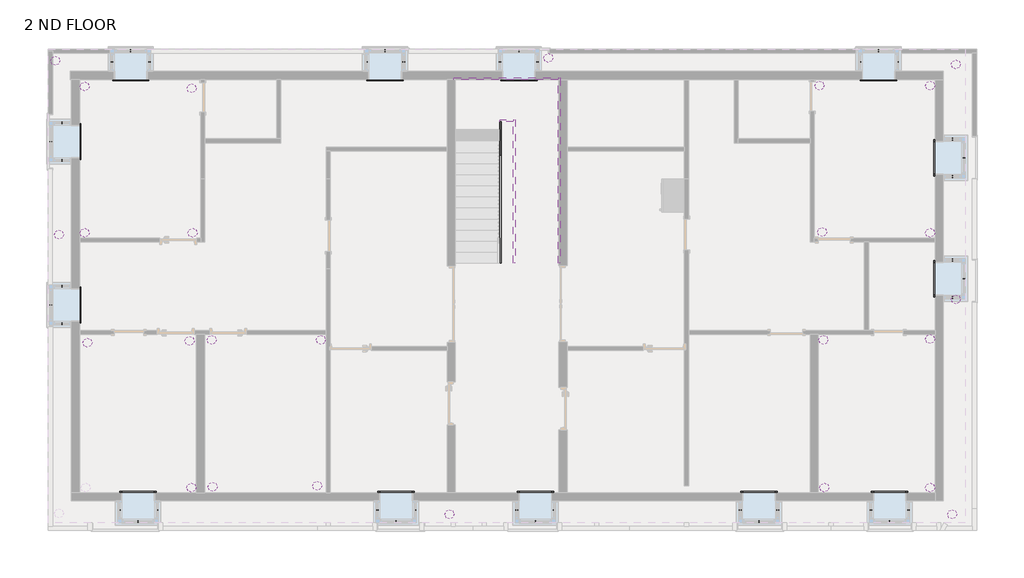
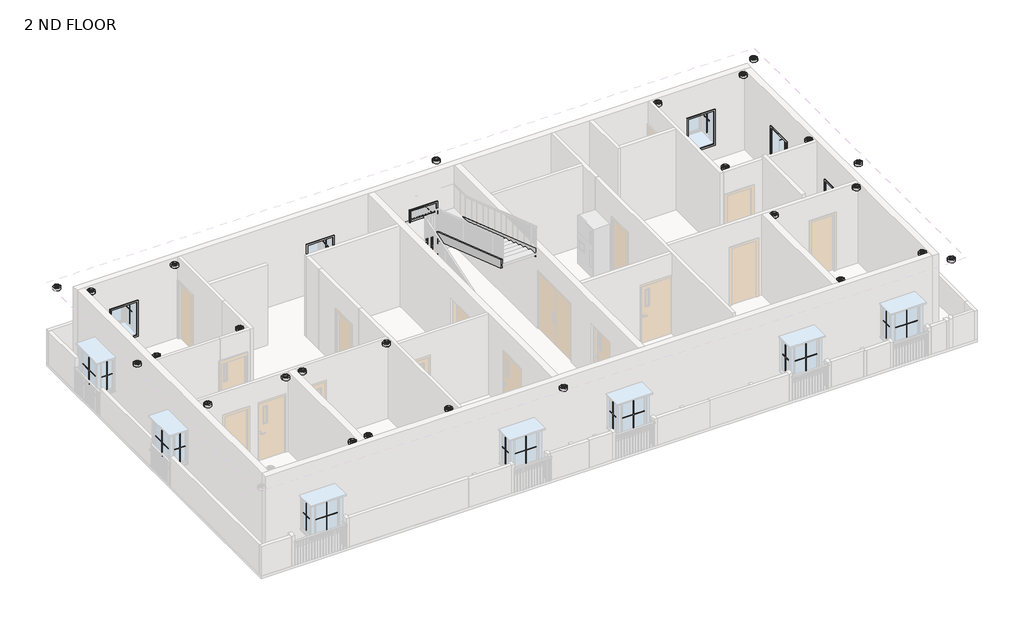
# One storey, part 7 of 7: 52 proxies, 26 light fixtures, 6 members.
"""IFC4 building model written with IfcOpenShell, lengths in millimetres."""

from ifc_helpers import new_model, si_unit, frame, origin, place, context, project, spatial, polyline, outline, extrude, transform, mapped, element, save
from components import muntin_pattern_2x2_muntin_pattern_2x2_95b57395, muntin_pattern_2x2_muntin_pattern_2x2_f03ab90d, trim_window_interior_flat_picture_frame_e50cf7ae, ceiling_light_flat_round_60w_120v_7c4c2a52

model = new_model("IFC4")

# Units and contexts
model_context = context("Model", 3, world=origin())
ifc_project = project(units=[si_unit("LENGTHUNIT", "METRE", prefix="MILLI")], contexts=[model_context])

# Site, building, storey
site = spatial("IfcSite", under=ifc_project)
building = spatial("IfcBuilding", under=site)
storey = spatial("IfcBuildingStorey", under=building, Name="2 ND FLOOR", Elevation=6400.8)

# Proxies
placement = place(None, origin())
muntin_pattern_2x2_muntin_pattern_2x2_shape = muntin_pattern_2x2_muntin_pattern_2x2_95b57395(model_context)
element("IfcBuildingElementProxy", 1, Name="Muntin Pattern_2x2 : Muntin Pattern_2x2", ObjectType="Muntin Pattern_2x2 : Muntin Pattern_2x2", at=placement, inside=storey, context=model_context, shape_type="MappedRepresentation", body=[
    mapped(muntin_pattern_2x2_muntin_pattern_2x2_shape, transform((-10814.9987925, 8428.7317329, 7131.05), x_axis=(1.0, 0.0, 0.0), y_axis=(0.0, 1.0, 0.0), z_axis=(0.0, 0.0, 1.0))),
])
element("IfcBuildingElementProxy", 2, Name="Muntin Pattern_2x2 : Muntin Pattern_2x2", ObjectType="Muntin Pattern_2x2 : Muntin Pattern_2x2", at=placement, inside=storey, context=model_context, shape_type="MappedRepresentation", body=[
    mapped(muntin_pattern_2x2_muntin_pattern_2x2_shape, transform((-3791.8987998, 8428.7317329, 7131.05), x_axis=(1.0, 0.0, 0.0), y_axis=(0.0, 1.0, 0.0), z_axis=(0.0, 0.0, 1.0))),
])
element("IfcBuildingElementProxy", 3, Name="Muntin Pattern_2x2 : Muntin Pattern_2x2", ObjectType="Muntin Pattern_2x2 : Muntin Pattern_2x2", at=placement, inside=storey, context=model_context, shape_type="MappedRepresentation", body=[
    mapped(muntin_pattern_2x2_muntin_pattern_2x2_shape, transform((-96.7067989, 8428.7317329, 7131.05), x_axis=(1.0, 0.0, 0.0), y_axis=(0.0, 1.0, 0.0), z_axis=(0.0, 0.0, 1.0))),
])
element("IfcBuildingElementProxy", 4, Name="Muntin Pattern_2x2 : Muntin Pattern_2x2", ObjectType="Muntin Pattern_2x2 : Muntin Pattern_2x2", at=placement, inside=storey, context=model_context, shape_type="MappedRepresentation", body=[
    mapped(muntin_pattern_2x2_muntin_pattern_2x2_shape, transform((9835.2012075, 8428.7317329, 7131.05), x_axis=(1.0, 0.0, 0.0), y_axis=(0.0, 1.0, 0.0), z_axis=(0.0, 0.0, 1.0))),
])
element("IfcBuildingElementProxy", 5, Name="Muntin Pattern_2x2 : Muntin Pattern_2x2", ObjectType="Muntin Pattern_2x2 : Muntin Pattern_2x2", at=placement, inside=storey, context=model_context, shape_type="MappedRepresentation", body=[
    mapped(muntin_pattern_2x2_muntin_pattern_2x2_shape, transform((-10611.7987958, -4582.4182193, 7131.05), x_axis=(-1.0, 0.0, 0.0), y_axis=(0.0, -1.0, 0.0), z_axis=(0.0, 0.0, 1.0))),
])
element("IfcBuildingElementProxy", 6, Name="Muntin Pattern_2x2 : Muntin Pattern_2x2", ObjectType="Muntin Pattern_2x2 : Muntin Pattern_2x2", at=placement, inside=storey, context=model_context, shape_type="MappedRepresentation", body=[
    mapped(muntin_pattern_2x2_muntin_pattern_2x2_shape, transform((-3487.0987998, -4582.4182193, 7131.05), x_axis=(-1.0, 0.0, 0.0), y_axis=(0.0, -1.0, 0.0), z_axis=(0.0, 0.0, 1.0))),
])
element("IfcBuildingElementProxy", 7, Name="Muntin Pattern_2x2 : Muntin Pattern_2x2", ObjectType="Muntin Pattern_2x2 : Muntin Pattern_2x2", at=placement, inside=storey, context=model_context, shape_type="MappedRepresentation", body=[
    mapped(muntin_pattern_2x2_muntin_pattern_2x2_shape, transform((360.4932011, -4582.4182193, 7131.05), x_axis=(-1.0, 0.0, 0.0), y_axis=(0.0, -1.0, 0.0), z_axis=(0.0, 0.0, 1.0))),
])
element("IfcBuildingElementProxy", 8, Name="Muntin Pattern_2x2 : Muntin Pattern_2x2", ObjectType="Muntin Pattern_2x2 : Muntin Pattern_2x2", at=placement, inside=storey, context=model_context, shape_type="MappedRepresentation", body=[
    mapped(muntin_pattern_2x2_muntin_pattern_2x2_shape, transform((6533.2012079, -4582.4182193, 7131.05), x_axis=(-1.0, 0.0, 0.0), y_axis=(0.0, -1.0, 0.0), z_axis=(0.0, 0.0, 1.0))),
])
element("IfcBuildingElementProxy", 9, Name="Muntin Pattern_2x2 : Muntin Pattern_2x2", ObjectType="Muntin Pattern_2x2 : Muntin Pattern_2x2", at=placement, inside=storey, context=model_context, shape_type="MappedRepresentation", body=[
    mapped(muntin_pattern_2x2_muntin_pattern_2x2_shape, transform((10140.0012075, -4582.4182193, 7131.05), x_axis=(-1.0, 0.0, 0.0), y_axis=(0.0, -1.0, 0.0), z_axis=(0.0, 0.0, 1.0))),
])
element("IfcBuildingElementProxy", 10, Name="Muntin Pattern_2x2 : Muntin Pattern_2x2", ObjectType="Muntin Pattern_2x2 : Muntin Pattern_2x2", at=placement, inside=storey, context=model_context, shape_type="MappedRepresentation", body=[
    mapped(muntin_pattern_2x2_muntin_pattern_2x2_shape, transform((12194.2262075, 2126.3567332, 7131.05), x_axis=(0.0, -1.0, 0.0), y_axis=(1.0, 0.0, 0.0), z_axis=(0.0, 0.0, 1.0))),
])
element("IfcBuildingElementProxy", 11, Name="Muntin Pattern_2x2 : Muntin Pattern_2x2", ObjectType="Muntin Pattern_2x2 : Muntin Pattern_2x2", at=placement, inside=storey, context=model_context, shape_type="MappedRepresentation", body=[
    mapped(muntin_pattern_2x2_muntin_pattern_2x2_shape, transform((12194.2262075, 5469.631733, 7131.05), x_axis=(0.0, -1.0, 0.0), y_axis=(1.0, 0.0, 0.0), z_axis=(0.0, 0.0, 1.0))),
])
element("IfcBuildingElementProxy", 12, Name="Muntin Pattern_2x2 : Muntin Pattern_2x2", ObjectType="Muntin Pattern_2x2 : Muntin Pattern_2x2", at=placement, inside=storey, context=model_context, shape_type="MappedRepresentation", body=[
    mapped(muntin_pattern_2x2_muntin_pattern_2x2_shape, transform((-13021.6237925, 1402.4567334, 7131.05), x_axis=(0.0, 1.0, 0.0), y_axis=(-1.0, 0.0, 0.0), z_axis=(0.0, 0.0, 1.0))),
])
element("IfcBuildingElementProxy", 13, Name="Muntin Pattern_2x2 : Muntin Pattern_2x2", ObjectType="Muntin Pattern_2x2 : Muntin Pattern_2x2", at=placement, inside=storey, context=model_context, shape_type="MappedRepresentation", body=[
    mapped(muntin_pattern_2x2_muntin_pattern_2x2_shape, transform((-13021.6237925, 5917.3067329, 7131.05), x_axis=(0.0, 1.0, 0.0), y_axis=(-1.0, 0.0, 0.0), z_axis=(0.0, 0.0, 1.0))),
])
muntin_pattern_2x2_muntin_pattern_2x2_2_shape = muntin_pattern_2x2_muntin_pattern_2x2_f03ab90d(model_context)
element("IfcBuildingElementProxy", 14, Name="Muntin Pattern_2x2 : Muntin Pattern_2x2", ObjectType="Muntin Pattern_2x2 : Muntin Pattern_2x2", at=placement, inside=storey, context=model_context, shape_type="MappedRepresentation", body=[
    mapped(muntin_pattern_2x2_muntin_pattern_2x2_2_shape, transform((-11332.5237925, 8114.4067329, 7131.05), x_axis=(0.0, -1.0, 0.0), y_axis=(1.0, 0.0, 0.0), z_axis=(0.0, 0.0, 1.0))),
])
element("IfcBuildingElementProxy", 15, Name="Muntin Pattern_2x2 : Muntin Pattern_2x2", ObjectType="Muntin Pattern_2x2 : Muntin Pattern_2x2", at=placement, inside=storey, context=model_context, shape_type="MappedRepresentation", body=[
    mapped(muntin_pattern_2x2_muntin_pattern_2x2_2_shape, transform((-10297.4737925, 8114.4067329, 7131.05), x_axis=(0.0, 1.0, 0.0), y_axis=(-1.0, 0.0, 0.0), z_axis=(0.0, 0.0, 1.0))),
])
element("IfcBuildingElementProxy", 16, Name="Muntin Pattern_2x2 : Muntin Pattern_2x2", ObjectType="Muntin Pattern_2x2 : Muntin Pattern_2x2", at=placement, inside=storey, context=model_context, shape_type="MappedRepresentation", body=[
    mapped(muntin_pattern_2x2_muntin_pattern_2x2_2_shape, transform((-4309.4237998, 8114.4067329, 7131.05), x_axis=(0.0, -1.0, 0.0), y_axis=(1.0, 0.0, 0.0), z_axis=(0.0, 0.0, 1.0))),
])
element("IfcBuildingElementProxy", 17, Name="Muntin Pattern_2x2 : Muntin Pattern_2x2", ObjectType="Muntin Pattern_2x2 : Muntin Pattern_2x2", at=placement, inside=storey, context=model_context, shape_type="MappedRepresentation", body=[
    mapped(muntin_pattern_2x2_muntin_pattern_2x2_2_shape, transform((-3274.3737998, 8114.4067329, 7131.05), x_axis=(0.0, 1.0, 0.0), y_axis=(-1.0, 0.0, 0.0), z_axis=(0.0, 0.0, 1.0))),
])
element("IfcBuildingElementProxy", 18, Name="Muntin Pattern_2x2 : Muntin Pattern_2x2", ObjectType="Muntin Pattern_2x2 : Muntin Pattern_2x2", at=placement, inside=storey, context=model_context, shape_type="MappedRepresentation", body=[
    mapped(muntin_pattern_2x2_muntin_pattern_2x2_2_shape, transform((-614.2317989, 8114.4067329, 7131.05), x_axis=(0.0, -1.0, 0.0), y_axis=(1.0, 0.0, 0.0), z_axis=(0.0, 0.0, 1.0))),
])
element("IfcBuildingElementProxy", 19, Name="Muntin Pattern_2x2 : Muntin Pattern_2x2", ObjectType="Muntin Pattern_2x2 : Muntin Pattern_2x2", at=placement, inside=storey, context=model_context, shape_type="MappedRepresentation", body=[
    mapped(muntin_pattern_2x2_muntin_pattern_2x2_2_shape, transform((420.8182011, 8114.4067329, 7131.05), x_axis=(0.0, 1.0, 0.0), y_axis=(-1.0, 0.0, 0.0), z_axis=(0.0, 0.0, 1.0))),
])
element("IfcBuildingElementProxy", 20, Name="Muntin Pattern_2x2 : Muntin Pattern_2x2", ObjectType="Muntin Pattern_2x2 : Muntin Pattern_2x2", at=placement, inside=storey, context=model_context, shape_type="MappedRepresentation", body=[
    mapped(muntin_pattern_2x2_muntin_pattern_2x2_2_shape, transform((9317.6762075, 8114.4067329, 7131.05), x_axis=(0.0, -1.0, 0.0), y_axis=(1.0, 0.0, 0.0), z_axis=(0.0, 0.0, 1.0))),
])
element("IfcBuildingElementProxy", 21, Name="Muntin Pattern_2x2 : Muntin Pattern_2x2", ObjectType="Muntin Pattern_2x2 : Muntin Pattern_2x2", at=placement, inside=storey, context=model_context, shape_type="MappedRepresentation", body=[
    mapped(muntin_pattern_2x2_muntin_pattern_2x2_2_shape, transform((10352.7262075, 8114.4067329, 7131.05), x_axis=(0.0, 1.0, 0.0), y_axis=(-1.0, 0.0, 0.0), z_axis=(0.0, 0.0, 1.0))),
])
element("IfcBuildingElementProxy", 22, Name="Muntin Pattern_2x2 : Muntin Pattern_2x2", ObjectType="Muntin Pattern_2x2 : Muntin Pattern_2x2", at=placement, inside=storey, context=model_context, shape_type="MappedRepresentation", body=[
    mapped(muntin_pattern_2x2_muntin_pattern_2x2_2_shape, transform((-10094.2737958, -4268.0932193, 7131.05), x_axis=(0.0, 1.0, 0.0), y_axis=(-1.0, 0.0, 0.0), z_axis=(0.0, 0.0, 1.0))),
])
element("IfcBuildingElementProxy", 23, Name="Muntin Pattern_2x2 : Muntin Pattern_2x2", ObjectType="Muntin Pattern_2x2 : Muntin Pattern_2x2", at=placement, inside=storey, context=model_context, shape_type="MappedRepresentation", body=[
    mapped(muntin_pattern_2x2_muntin_pattern_2x2_2_shape, transform((-11129.3237958, -4268.0932193, 7131.05), x_axis=(0.0, -1.0, 0.0), y_axis=(1.0, 0.0, 0.0), z_axis=(0.0, 0.0, 1.0))),
])
element("IfcBuildingElementProxy", 24, Name="Muntin Pattern_2x2 : Muntin Pattern_2x2", ObjectType="Muntin Pattern_2x2 : Muntin Pattern_2x2", at=placement, inside=storey, context=model_context, shape_type="MappedRepresentation", body=[
    mapped(muntin_pattern_2x2_muntin_pattern_2x2_2_shape, transform((-2969.5737998, -4268.0932193, 7131.05), x_axis=(0.0, 1.0, 0.0), y_axis=(-1.0, 0.0, 0.0), z_axis=(0.0, 0.0, 1.0))),
])
element("IfcBuildingElementProxy", 25, Name="Muntin Pattern_2x2 : Muntin Pattern_2x2", ObjectType="Muntin Pattern_2x2 : Muntin Pattern_2x2", at=placement, inside=storey, context=model_context, shape_type="MappedRepresentation", body=[
    mapped(muntin_pattern_2x2_muntin_pattern_2x2_2_shape, transform((-4004.6237998, -4268.0932193, 7131.05), x_axis=(0.0, -1.0, 0.0), y_axis=(1.0, 0.0, 0.0), z_axis=(0.0, 0.0, 1.0))),
])
element("IfcBuildingElementProxy", 26, Name="Muntin Pattern_2x2 : Muntin Pattern_2x2", ObjectType="Muntin Pattern_2x2 : Muntin Pattern_2x2", at=placement, inside=storey, context=model_context, shape_type="MappedRepresentation", body=[
    mapped(muntin_pattern_2x2_muntin_pattern_2x2_2_shape, transform((878.0182011, -4268.0932193, 7131.05), x_axis=(0.0, 1.0, 0.0), y_axis=(-1.0, 0.0, 0.0), z_axis=(0.0, 0.0, 1.0))),
])
element("IfcBuildingElementProxy", 27, Name="Muntin Pattern_2x2 : Muntin Pattern_2x2", ObjectType="Muntin Pattern_2x2 : Muntin Pattern_2x2", at=placement, inside=storey, context=model_context, shape_type="MappedRepresentation", body=[
    mapped(muntin_pattern_2x2_muntin_pattern_2x2_2_shape, transform((-157.0317989, -4268.0932193, 7131.05), x_axis=(0.0, -1.0, 0.0), y_axis=(1.0, 0.0, 0.0), z_axis=(0.0, 0.0, 1.0))),
])
element("IfcBuildingElementProxy", 28, Name="Muntin Pattern_2x2 : Muntin Pattern_2x2", ObjectType="Muntin Pattern_2x2 : Muntin Pattern_2x2", at=placement, inside=storey, context=model_context, shape_type="MappedRepresentation", body=[
    mapped(muntin_pattern_2x2_muntin_pattern_2x2_2_shape, transform((7050.7262079, -4268.0932193, 7131.05), x_axis=(0.0, 1.0, 0.0), y_axis=(-1.0, 0.0, 0.0), z_axis=(0.0, 0.0, 1.0))),
])
element("IfcBuildingElementProxy", 29, Name="Muntin Pattern_2x2 : Muntin Pattern_2x2", ObjectType="Muntin Pattern_2x2 : Muntin Pattern_2x2", at=placement, inside=storey, context=model_context, shape_type="MappedRepresentation", body=[
    mapped(muntin_pattern_2x2_muntin_pattern_2x2_2_shape, transform((6015.6762079, -4268.0932193, 7131.05), x_axis=(0.0, -1.0, 0.0), y_axis=(1.0, 0.0, 0.0), z_axis=(0.0, 0.0, 1.0))),
])
element("IfcBuildingElementProxy", 30, Name="Muntin Pattern_2x2 : Muntin Pattern_2x2", ObjectType="Muntin Pattern_2x2 : Muntin Pattern_2x2", at=placement, inside=storey, context=model_context, shape_type="MappedRepresentation", body=[
    mapped(muntin_pattern_2x2_muntin_pattern_2x2_2_shape, transform((10657.5262075, -4268.0932193, 7131.05), x_axis=(0.0, 1.0, 0.0), y_axis=(-1.0, 0.0, 0.0), z_axis=(0.0, 0.0, 1.0))),
])
element("IfcBuildingElementProxy", 31, Name="Muntin Pattern_2x2 : Muntin Pattern_2x2", ObjectType="Muntin Pattern_2x2 : Muntin Pattern_2x2", at=placement, inside=storey, context=model_context, shape_type="MappedRepresentation", body=[
    mapped(muntin_pattern_2x2_muntin_pattern_2x2_2_shape, transform((9622.4762075, -4268.0932193, 7131.05), x_axis=(0.0, -1.0, 0.0), y_axis=(1.0, 0.0, 0.0), z_axis=(0.0, 0.0, 1.0))),
])
element("IfcBuildingElementProxy", 32, Name="Muntin Pattern_2x2 : Muntin Pattern_2x2", ObjectType="Muntin Pattern_2x2 : Muntin Pattern_2x2", at=placement, inside=storey, context=model_context, shape_type="MappedRepresentation", body=[
    mapped(muntin_pattern_2x2_muntin_pattern_2x2_2_shape, transform((11879.9012075, 2643.8817332, 7131.05), x_axis=(-1.0, 0.0, 0.0), y_axis=(0.0, -1.0, 0.0), z_axis=(0.0, 0.0, 1.0))),
])
element("IfcBuildingElementProxy", 33, Name="Muntin Pattern_2x2 : Muntin Pattern_2x2", ObjectType="Muntin Pattern_2x2 : Muntin Pattern_2x2", at=placement, inside=storey, context=model_context, shape_type="MappedRepresentation", body=[
    mapped(muntin_pattern_2x2_muntin_pattern_2x2_2_shape, transform((11879.9012075, 1608.8317332, 7131.05), x_axis=(1.0, 0.0, 0.0), y_axis=(0.0, 1.0, 0.0), z_axis=(0.0, 0.0, 1.0))),
])
element("IfcBuildingElementProxy", 34, Name="Muntin Pattern_2x2 : Muntin Pattern_2x2", ObjectType="Muntin Pattern_2x2 : Muntin Pattern_2x2", at=placement, inside=storey, context=model_context, shape_type="MappedRepresentation", body=[
    mapped(muntin_pattern_2x2_muntin_pattern_2x2_2_shape, transform((11879.9012075, 5987.156733, 7131.05), x_axis=(-1.0, 0.0, 0.0), y_axis=(0.0, -1.0, 0.0), z_axis=(0.0, 0.0, 1.0))),
])
element("IfcBuildingElementProxy", 35, Name="Muntin Pattern_2x2 : Muntin Pattern_2x2", ObjectType="Muntin Pattern_2x2 : Muntin Pattern_2x2", at=placement, inside=storey, context=model_context, shape_type="MappedRepresentation", body=[
    mapped(muntin_pattern_2x2_muntin_pattern_2x2_2_shape, transform((11879.9012075, 4952.106733, 7131.05), x_axis=(1.0, 0.0, 0.0), y_axis=(0.0, 1.0, 0.0), z_axis=(0.0, 0.0, 1.0))),
])
element("IfcBuildingElementProxy", 36, Name="Muntin Pattern_2x2 : Muntin Pattern_2x2", ObjectType="Muntin Pattern_2x2 : Muntin Pattern_2x2", at=placement, inside=storey, context=model_context, shape_type="MappedRepresentation", body=[
    mapped(muntin_pattern_2x2_muntin_pattern_2x2_2_shape, transform((-12707.2987925, 884.9317334, 7131.05), x_axis=(1.0, 0.0, 0.0), y_axis=(0.0, 1.0, 0.0), z_axis=(0.0, 0.0, 1.0))),
])
element("IfcBuildingElementProxy", 37, Name="Muntin Pattern_2x2 : Muntin Pattern_2x2", ObjectType="Muntin Pattern_2x2 : Muntin Pattern_2x2", at=placement, inside=storey, context=model_context, shape_type="MappedRepresentation", body=[
    mapped(muntin_pattern_2x2_muntin_pattern_2x2_2_shape, transform((-12707.2987925, 1919.9817334, 7131.05), x_axis=(-1.0, 0.0, 0.0), y_axis=(0.0, -1.0, 0.0), z_axis=(0.0, 0.0, 1.0))),
])
element("IfcBuildingElementProxy", 38, Name="Muntin Pattern_2x2 : Muntin Pattern_2x2", ObjectType="Muntin Pattern_2x2 : Muntin Pattern_2x2", at=placement, inside=storey, context=model_context, shape_type="MappedRepresentation", body=[
    mapped(muntin_pattern_2x2_muntin_pattern_2x2_2_shape, transform((-12707.2987925, 5399.7817329, 7131.05), x_axis=(1.0, 0.0, 0.0), y_axis=(0.0, 1.0, 0.0), z_axis=(0.0, 0.0, 1.0))),
])
element("IfcBuildingElementProxy", 39, Name="Muntin Pattern_2x2 : Muntin Pattern_2x2", ObjectType="Muntin Pattern_2x2 : Muntin Pattern_2x2", at=placement, inside=storey, context=model_context, shape_type="MappedRepresentation", body=[
    mapped(muntin_pattern_2x2_muntin_pattern_2x2_2_shape, transform((-12707.2987925, 6434.8317329, 7131.05), x_axis=(-1.0, 0.0, 0.0), y_axis=(0.0, -1.0, 0.0), z_axis=(0.0, 0.0, 1.0))),
])
trim_window_interior_flat_picture_frame_shape = trim_window_interior_flat_picture_frame_e50cf7ae(model_context)
element("IfcBuildingElementProxy", 40, Name="Trim-Window-Interior-Flat : Picture Frame", ObjectType="Trim-Window-Interior-Flat : Picture Frame", at=placement, inside=storey, context=model_context, shape_type="MappedRepresentation", body=[
    mapped(trim_window_interior_flat_picture_frame_shape, transform((-10814.9987925, 7631.8067329, 8280.4), x_axis=(1.0, 0.0, 0.0), y_axis=(0.0, 0.0, 1.0), z_axis=(0.0, -1.0, 0.0))),
])
element("IfcBuildingElementProxy", 41, Name="Trim-Window-Interior-Flat : Picture Frame", ObjectType="Trim-Window-Interior-Flat : Picture Frame", at=placement, inside=storey, context=model_context, shape_type="MappedRepresentation", body=[
    mapped(trim_window_interior_flat_picture_frame_shape, transform((-3791.8987998, 7631.8067329, 8280.4), x_axis=(1.0, 0.0, 0.0), y_axis=(0.0, 0.0, 1.0), z_axis=(0.0, -1.0, 0.0))),
])
element("IfcBuildingElementProxy", 42, Name="Trim-Window-Interior-Flat : Picture Frame", ObjectType="Trim-Window-Interior-Flat : Picture Frame", at=placement, inside=storey, context=model_context, shape_type="MappedRepresentation", body=[
    mapped(trim_window_interior_flat_picture_frame_shape, transform((-96.7067989, 7631.8067329, 8280.4), x_axis=(1.0, 0.0, 0.0), y_axis=(0.0, 0.0, 1.0), z_axis=(0.0, -1.0, 0.0))),
])
element("IfcBuildingElementProxy", 43, Name="Trim-Window-Interior-Flat : Picture Frame", ObjectType="Trim-Window-Interior-Flat : Picture Frame", at=placement, inside=storey, context=model_context, shape_type="MappedRepresentation", body=[
    mapped(trim_window_interior_flat_picture_frame_shape, transform((9835.2012075, 7631.8067329, 8280.4), x_axis=(1.0, 0.0, 0.0), y_axis=(0.0, 0.0, 1.0), z_axis=(0.0, -1.0, 0.0))),
])
element("IfcBuildingElementProxy", 44, Name="Trim-Window-Interior-Flat : Picture Frame", ObjectType="Trim-Window-Interior-Flat : Picture Frame", at=placement, inside=storey, context=model_context, shape_type="MappedRepresentation", body=[
    mapped(trim_window_interior_flat_picture_frame_shape, transform((-10611.7987958, -3785.4932193, 8280.4), x_axis=(-1.0, 0.0, 0.0), y_axis=(0.0, 0.0, 1.0), z_axis=(0.0, 1.0, 0.0))),
])
element("IfcBuildingElementProxy", 45, Name="Trim-Window-Interior-Flat : Picture Frame", ObjectType="Trim-Window-Interior-Flat : Picture Frame", at=placement, inside=storey, context=model_context, shape_type="MappedRepresentation", body=[
    mapped(trim_window_interior_flat_picture_frame_shape, transform((-3487.0987998, -3785.4932193, 8280.4), x_axis=(-1.0, 0.0, 0.0), y_axis=(0.0, 0.0, 1.0), z_axis=(0.0, 1.0, 0.0))),
])
element("IfcBuildingElementProxy", 46, Name="Trim-Window-Interior-Flat : Picture Frame", ObjectType="Trim-Window-Interior-Flat : Picture Frame", at=placement, inside=storey, context=model_context, shape_type="MappedRepresentation", body=[
    mapped(trim_window_interior_flat_picture_frame_shape, transform((360.4932011, -3785.4932193, 8280.4), x_axis=(-1.0, 0.0, 0.0), y_axis=(0.0, 0.0, 1.0), z_axis=(0.0, 1.0, 0.0))),
])
element("IfcBuildingElementProxy", 47, Name="Trim-Window-Interior-Flat : Picture Frame", ObjectType="Trim-Window-Interior-Flat : Picture Frame", at=placement, inside=storey, context=model_context, shape_type="MappedRepresentation", body=[
    mapped(trim_window_interior_flat_picture_frame_shape, transform((6533.2012079, -3785.4932193, 8280.4), x_axis=(-1.0, 0.0, 0.0), y_axis=(0.0, 0.0, 1.0), z_axis=(0.0, 1.0, 0.0))),
])
element("IfcBuildingElementProxy", 48, Name="Trim-Window-Interior-Flat : Picture Frame", ObjectType="Trim-Window-Interior-Flat : Picture Frame", at=placement, inside=storey, context=model_context, shape_type="MappedRepresentation", body=[
    mapped(trim_window_interior_flat_picture_frame_shape, transform((10140.0012075, -3785.4932193, 8280.4), x_axis=(-1.0, 0.0, 0.0), y_axis=(0.0, 0.0, 1.0), z_axis=(0.0, 1.0, 0.0))),
])
element("IfcBuildingElementProxy", 49, Name="Trim-Window-Interior-Flat : Picture Frame", ObjectType="Trim-Window-Interior-Flat : Picture Frame", at=placement, inside=storey, context=model_context, shape_type="MappedRepresentation", body=[
    mapped(trim_window_interior_flat_picture_frame_shape, transform((11397.3012075, 2126.3567332, 8280.4), x_axis=(0.0, -1.0, 0.0), y_axis=(0.0, 0.0, 1.0), z_axis=(-1.0, 0.0, 0.0))),
])
element("IfcBuildingElementProxy", 50, Name="Trim-Window-Interior-Flat : Picture Frame", ObjectType="Trim-Window-Interior-Flat : Picture Frame", at=placement, inside=storey, context=model_context, shape_type="MappedRepresentation", body=[
    mapped(trim_window_interior_flat_picture_frame_shape, transform((11397.3012075, 5469.631733, 8280.4), x_axis=(0.0, -1.0, 0.0), y_axis=(0.0, 0.0, 1.0), z_axis=(-1.0, 0.0, 0.0))),
])
element("IfcBuildingElementProxy", 51, Name="Trim-Window-Interior-Flat : Picture Frame", ObjectType="Trim-Window-Interior-Flat : Picture Frame", at=placement, inside=storey, context=model_context, shape_type="MappedRepresentation", body=[
    mapped(trim_window_interior_flat_picture_frame_shape, transform((-12224.6987925, 1402.4567334, 8280.4), x_axis=(0.0, 1.0, 0.0), y_axis=(0.0, 0.0, 1.0), z_axis=(1.0, 0.0, 0.0))),
])
element("IfcBuildingElementProxy", 52, Name="Trim-Window-Interior-Flat : Picture Frame", ObjectType="Trim-Window-Interior-Flat : Picture Frame", at=placement, inside=storey, context=model_context, shape_type="MappedRepresentation", body=[
    mapped(trim_window_interior_flat_picture_frame_shape, transform((-12224.6987925, 5917.3067329, 8280.4), x_axis=(0.0, 1.0, 0.0), y_axis=(0.0, 0.0, 1.0), z_axis=(1.0, 0.0, 0.0))),
])

# Light fixtures
ceiling_light_flat_round_60w_120v_shape = ceiling_light_flat_round_60w_120v_7c4c2a52(model_context)
element("IfcLightFixture", 53, ObjectType="Ceiling Light - Flat Round : 60W - 120V", at=placement, inside=storey, context=model_context, shape_type="MappedRepresentation", body=[
    mapped(ceiling_light_flat_round_60w_120v_shape, transform((-12897.7987925, 8152.5067329, 7010.4), x_axis=(1.0, 0.0, 0.0), y_axis=(0.0, 1.0, 0.0), z_axis=(0.0, 0.0, 1.0))),
])
element("IfcLightFixture", 54, ObjectType="Ceiling Light - Flat Round : 60W - 120V", at=placement, inside=storey, context=model_context, shape_type="MappedRepresentation", body=[
    mapped(ceiling_light_flat_round_60w_120v_shape, transform((-12796.1987925, 3345.5567332, 7010.4), x_axis=(1.0, 0.0, 0.0), y_axis=(0.0, 1.0, 0.0), z_axis=(0.0, 0.0, 1.0))),
])
element("IfcLightFixture", 55, ObjectType="Ceiling Light - Flat Round : 60W - 120V", at=placement, inside=storey, context=model_context, shape_type="MappedRepresentation", body=[
    mapped(ceiling_light_flat_round_60w_120v_shape, transform((-2013.8987998, -4382.3932193, 7010.4), x_axis=(1.0, 0.0, 0.0), y_axis=(0.0, 1.0, 0.0), z_axis=(0.0, 0.0, 1.0))),
])
element("IfcLightFixture", 56, ObjectType="Ceiling Light - Flat Round : 60W - 120V", at=placement, inside=storey, context=model_context, shape_type="MappedRepresentation", body=[
    mapped(ceiling_light_flat_round_60w_120v_shape, transform((11867.2012075, -4382.3932193, 7010.4), x_axis=(1.0, 0.0, 0.0), y_axis=(0.0, 1.0, 0.0), z_axis=(0.0, 0.0, 1.0))),
])
element("IfcLightFixture", 57, ObjectType="Ceiling Light - Flat Round : 60W - 120V", at=placement, inside=storey, context=model_context, shape_type="MappedRepresentation", body=[
    mapped(ceiling_light_flat_round_60w_120v_shape, transform((11968.8012075, 1554.8567334, 7010.4), x_axis=(1.0, 0.0, 0.0), y_axis=(0.0, 1.0, 0.0), z_axis=(0.0, 0.0, 1.0))),
])
element("IfcLightFixture", 58, ObjectType="Ceiling Light - Flat Round : 60W - 120V", at=placement, inside=storey, context=model_context, shape_type="MappedRepresentation", body=[
    mapped(ceiling_light_flat_round_60w_120v_shape, transform((11968.8012075, 8050.9067329, 7010.4), x_axis=(1.0, 0.0, 0.0), y_axis=(0.0, 1.0, 0.0), z_axis=(0.0, 0.0, 1.0))),
])
element("IfcLightFixture", 59, ObjectType="Ceiling Light - Flat Round : 60W - 120V", at=placement, inside=storey, context=model_context, shape_type="MappedRepresentation", body=[
    mapped(ceiling_light_flat_round_60w_120v_shape, transform((716.0932011, 8228.7067329, 7010.4), x_axis=(1.0, 0.0, 0.0), y_axis=(0.0, 1.0, 0.0), z_axis=(0.0, 0.0, 1.0))),
])
element("IfcLightFixture", 60, ObjectType="Ceiling Light - Flat Round : 60W - 120V", at=placement, inside=storey, context=model_context, shape_type="MappedRepresentation", body=[
    mapped(ceiling_light_flat_round_60w_120v_shape, transform((8203.2512079, 7466.7067329, 7010.4), x_axis=(1.0, 0.0, 0.0), y_axis=(0.0, 1.0, 0.0), z_axis=(0.0, 0.0, 1.0))),
])
element("IfcLightFixture", 61, ObjectType="Ceiling Light - Flat Round : 60W - 120V", at=placement, inside=storey, context=model_context, shape_type="MappedRepresentation", body=[
    mapped(ceiling_light_flat_round_60w_120v_shape, transform((11257.6012075, 7466.7067329, 7010.4), x_axis=(1.0, 0.0, 0.0), y_axis=(0.0, 1.0, 0.0), z_axis=(0.0, 0.0, 1.0))),
])
element("IfcLightFixture", 62, ObjectType="Ceiling Light - Flat Round : 60W - 120V", at=placement, inside=storey, context=model_context, shape_type="MappedRepresentation", body=[
    mapped(ceiling_light_flat_round_60w_120v_shape, transform((8279.4512079, 3421.7567332, 7010.4), x_axis=(1.0, 0.0, 0.0), y_axis=(0.0, 1.0, 0.0), z_axis=(0.0, 0.0, 1.0))),
])
element("IfcLightFixture", 63, ObjectType="Ceiling Light - Flat Round : 60W - 120V", at=placement, inside=storey, context=model_context, shape_type="MappedRepresentation", body=[
    mapped(ceiling_light_flat_round_60w_120v_shape, transform((11257.6012075, 3396.3567332, 7010.4), x_axis=(1.0, 0.0, 0.0), y_axis=(0.0, 1.0, 0.0), z_axis=(0.0, 0.0, 1.0))),
])
element("IfcLightFixture", 64, ObjectType="Ceiling Light - Flat Round : 60W - 120V", at=placement, inside=storey, context=model_context, shape_type="MappedRepresentation", body=[
    mapped(ceiling_light_flat_round_60w_120v_shape, transform((8311.2012079, 437.2567334, 7010.4), x_axis=(1.0, 0.0, 0.0), y_axis=(0.0, 1.0, 0.0), z_axis=(0.0, 0.0, 1.0))),
])
element("IfcLightFixture", 65, ObjectType="Ceiling Light - Flat Round : 60W - 120V", at=placement, inside=storey, context=model_context, shape_type="MappedRepresentation", body=[
    mapped(ceiling_light_flat_round_60w_120v_shape, transform((11257.6012075, 462.6567334, 7010.4), x_axis=(1.0, 0.0, 0.0), y_axis=(0.0, 1.0, 0.0), z_axis=(0.0, 0.0, 1.0))),
])
element("IfcLightFixture", 66, ObjectType="Ceiling Light - Flat Round : 60W - 120V", at=placement, inside=storey, context=model_context, shape_type="MappedRepresentation", body=[
    mapped(ceiling_light_flat_round_60w_120v_shape, transform((8336.6012079, -3645.7932193, 7010.4), x_axis=(1.0, 0.0, 0.0), y_axis=(0.0, 1.0, 0.0), z_axis=(0.0, 0.0, 1.0))),
])
element("IfcLightFixture", 67, ObjectType="Ceiling Light - Flat Round : 60W - 120V", at=placement, inside=storey, context=model_context, shape_type="MappedRepresentation", body=[
    mapped(ceiling_light_flat_round_60w_120v_shape, transform((11257.6012075, -3645.7932193, 7010.4), x_axis=(1.0, 0.0, 0.0), y_axis=(0.0, 1.0, 0.0), z_axis=(0.0, 0.0, 1.0))),
])
element("IfcLightFixture", 68, ObjectType="Ceiling Light - Flat Round : 60W - 120V", at=placement, inside=storey, context=model_context, shape_type="MappedRepresentation", body=[
    mapped(ceiling_light_flat_round_60w_120v_shape, transform((-12008.7987925, 361.0567334, 7010.4), x_axis=(1.0, 0.0, 0.0), y_axis=(0.0, 1.0, 0.0), z_axis=(0.0, 0.0, 1.0))),
])
element("IfcLightFixture", 69, ObjectType="Ceiling Light - Flat Round : 60W - 120V", at=placement, inside=storey, context=model_context, shape_type="MappedRepresentation", body=[
    mapped(ceiling_light_flat_round_60w_120v_shape, transform((-9189.3987992, 411.8567334, 7010.4), x_axis=(1.0, 0.0, 0.0), y_axis=(0.0, 1.0, 0.0), z_axis=(0.0, 0.0, 1.0))),
])
element("IfcLightFixture", 70, ObjectType="Ceiling Light - Flat Round : 60W - 120V", at=placement, inside=storey, context=model_context, shape_type="MappedRepresentation", body=[
    mapped(ceiling_light_flat_round_60w_120v_shape, transform((-9138.5987992, -3645.7932193, 7010.4), x_axis=(1.0, 0.0, 0.0), y_axis=(0.0, 1.0, 0.0), z_axis=(0.0, 0.0, 1.0))),
])
element("IfcLightFixture", 71, ObjectType="Ceiling Light - Flat Round : 60W - 120V", at=placement, inside=storey, context=model_context, shape_type="MappedRepresentation", body=[
    mapped(ceiling_light_flat_round_60w_120v_shape, transform((-8579.7987992, 437.2567334, 7010.4), x_axis=(1.0, 0.0, 0.0), y_axis=(0.0, 1.0, 0.0), z_axis=(0.0, 0.0, 1.0))),
])
element("IfcLightFixture", 72, ObjectType="Ceiling Light - Flat Round : 60W - 120V", at=placement, inside=storey, context=model_context, shape_type="MappedRepresentation", body=[
    mapped(ceiling_light_flat_round_60w_120v_shape, transform((-5563.5487995, 437.2567334, 7010.4), x_axis=(1.0, 0.0, 0.0), y_axis=(0.0, 1.0, 0.0), z_axis=(0.0, 0.0, 1.0))),
])
element("IfcLightFixture", 73, ObjectType="Ceiling Light - Flat Round : 60W - 120V", at=placement, inside=storey, context=model_context, shape_type="MappedRepresentation", body=[
    mapped(ceiling_light_flat_round_60w_120v_shape, transform((-8554.3987992, -3620.3932193, 7010.4), x_axis=(1.0, 0.0, 0.0), y_axis=(0.0, 1.0, 0.0), z_axis=(0.0, 0.0, 1.0))),
])
element("IfcLightFixture", 74, ObjectType="Ceiling Light - Flat Round : 60W - 120V", at=placement, inside=storey, context=model_context, shape_type="MappedRepresentation", body=[
    mapped(ceiling_light_flat_round_60w_120v_shape, transform((-5665.1487995, -3594.9932193, 7010.4), x_axis=(1.0, 0.0, 0.0), y_axis=(0.0, 1.0, 0.0), z_axis=(0.0, 0.0, 1.0))),
])
element("IfcLightFixture", 75, ObjectType="Ceiling Light - Flat Round : 60W - 120V", at=placement, inside=storey, context=model_context, shape_type="MappedRepresentation", body=[
    mapped(ceiling_light_flat_round_60w_120v_shape, transform((-12084.9987925, 7441.3067329, 7010.4), x_axis=(1.0, 0.0, 0.0), y_axis=(0.0, 1.0, 0.0), z_axis=(0.0, 0.0, 1.0))),
])
element("IfcLightFixture", 76, ObjectType="Ceiling Light - Flat Round : 60W - 120V", at=placement, inside=storey, context=model_context, shape_type="MappedRepresentation", body=[
    mapped(ceiling_light_flat_round_60w_120v_shape, transform((-9132.2487992, 7390.5067329, 7010.4), x_axis=(1.0, 0.0, 0.0), y_axis=(0.0, 1.0, 0.0), z_axis=(0.0, 0.0, 1.0))),
])
element("IfcLightFixture", 77, ObjectType="Ceiling Light - Flat Round : 60W - 120V", at=placement, inside=storey, context=model_context, shape_type="MappedRepresentation", body=[
    mapped(ceiling_light_flat_round_60w_120v_shape, transform((-12084.9987925, 3396.3567332, 7010.4), x_axis=(1.0, 0.0, 0.0), y_axis=(0.0, 1.0, 0.0), z_axis=(0.0, 0.0, 1.0))),
])
element("IfcLightFixture", 78, ObjectType="Ceiling Light - Flat Round : 60W - 120V", at=placement, inside=storey, context=model_context, shape_type="MappedRepresentation", body=[
    mapped(ceiling_light_flat_round_60w_120v_shape, transform((-9106.8487992, 3396.3567332, 7010.4), x_axis=(1.0, 0.0, 0.0), y_axis=(0.0, 1.0, 0.0), z_axis=(0.0, 0.0, 1.0))),
])

# Members
element("IfcMember", 79, ObjectType="Stringer - 2\" Width", at=placement, inside=storey, context=model_context, shape_type="SweptSolid", body=[
    extrude(outline(polyline([(2564.5067329, 6400.8), (2564.5067329, 6594.038056), (6486.7524627, 7924.8), (7435.4093802, 7924.8), (2943.6199065, 6400.8), (2564.5067329, 6400.8)])), frame((-1899.5987998, 0.0, 0.0), z_axis=(1.0, 0.0, 0.0), x_axis=(0.0, 1.0, 0.0)), (0.0, 0.0, 1.0), 50.8),
])
element("IfcMember", 80, ObjectType="Stringer - 2\" Width", at=placement, inside=storey, context=model_context, shape_type="SweptSolid", body=[
    extrude(outline(polyline([(-1899.5987998, 7631.8067329), (-1899.5987998, 7682.6067329), (996.0012002, 7682.6067329), (996.0012002, 7631.8067329), (-1899.5987998, 7631.8067329)])), frame((0.0, 0.0, 7620.0), z_axis=(0.0, 0.0, 1.0), x_axis=(1.0, 0.0, 0.0)), (0.0, 0.0, 1.0), 304.8),
])
element("IfcMember", 81, ObjectType="Stringer - 2\" Width", at=placement, inside=storey, context=model_context, shape_type="SweptSolid", body=[
    extrude(outline(polyline([(7682.6067329, 7649.725556), (7682.6067329, 7620.0), (6821.5619804, 7620.0), (2564.5067329, 9064.3580304), (2564.5067329, 9386.2237702), (7682.6067329, 7649.725556)])), frame((996.0012002, 0.0, 0.0), z_axis=(1.0, 0.0, 0.0), x_axis=(0.0, 1.0, 0.0)), (0.0, 0.0, 1.0), 50.8),
])
element("IfcMember", 82, ObjectType="Stringer - 2\" Width", at=placement, inside=storey, context=model_context, shape_type="SweptSolid", body=[
    extrude(outline(polyline([(2564.5067329, 6400.8), (2564.5067329, 6594.038056), (6476.1067329, 7921.188056), (6476.1067329, 7599.3223161), (2943.6199065, 6400.8), (2564.5067329, 6400.8)])), frame((-629.5987998, 0.0, 0.0), z_axis=(1.0, 0.0, 0.0), x_axis=(0.0, 1.0, 0.0)), (0.0, 0.0, 1.0), 50.8),
])
element("IfcMember", 83, ObjectType="Stringer - 2\" Width", at=placement, inside=storey, context=model_context, shape_type="SweptSolid", body=[
    extrude(outline(polyline([(-629.5987998, 6476.1067329), (-629.5987998, 6526.9067329), (-248.5987915, 6526.9067329), (-248.5987915, 6476.1067329), (-629.5987998, 6476.1067329)])), frame((0.0, 0.0, 7620.0), z_axis=(0.0, 0.0, 1.0), x_axis=(1.0, 0.0, 0.0)), (0.0, 0.0, 1.0), 304.8),
])
element("IfcMember", 84, ObjectType="Stringer - 2\" Width", at=placement, inside=storey, context=model_context, shape_type="SweptSolid", body=[
    extrude(outline(polyline([(6526.9067329, 8041.838056), (6526.9067329, 7719.9723161), (2564.5067329, 9064.3580304), (2564.5067329, 9386.2237702), (6526.9067329, 8041.838056)])), frame((-248.5987915, 0.0, 0.0), z_axis=(1.0, 0.0, 0.0), x_axis=(0.0, 1.0, 0.0)), (0.0, 0.0, 1.0), 50.8),
])

save(model, "model.ifc")

# Revit data of these elements
# Type "Muntin Pattern_2x2 : Muntin Pattern_2x2"
#   Width [instance default] = 4' - 0"
#   Thickness = 0' - 0 1/2"
#   Height [instance default] = 4' - 0"
#   Distance = 0' - 0 3/4"
#   Interior Material [instance default] = none
#   Exterior Material [instance default] = none
#   Default Elevation = 0
# Type "Trim-Window-Interior-Flat : Picture Frame"
#   Trim Thickness_Picture Frame = 0' - 1 1/4"
#   Trim Width = 0' - 2 1/4"
#   Trim Thickness_with Sill = 0' - 0 3/4"
#   Sill Thickness = 0' - 1 1/4"
#   Opening Width [instance default] = 2' - 0"
#   Opening Height [instance default] = 3' - 0"
#   Default Elevation = 4' - 0"
#   Sill = no
#   Picture Frame = yes
#   Trim Material [instance default] = none
# Type "Ceiling Light - Flat Round : 60W - 120V"
#   Lamp = "A-19"
#   Assembly Code = "D5020220"
#   Wattage = 60 W
#   built-in parameter 1150110 = 1 (stored number, unit not read)
#   built-in parameter 1114217 = 1 (stored number, unit not read)
#   built-in parameter 1150109 = 1 (stored number, unit not read)
#   built-in parameter 1150113 = 1 (stored number, unit not read)
#   built-in parameter 1150115 = 1 (stored number, unit not read)
#   built-in parameter 1150105 = 272.155 (stored number, unit not read)
#   Light Source Symbol Size = 2' - 0"
#   built-in parameter 1150112 = 1 (stored number, unit not read)
#   built-in parameter 1150114 = 1 (stored number, unit not read)
#   built-in parameter 1150107 = 2800 (stored number, unit not read)
#   built-in parameter 1150106 = 2.72155 (stored number, unit not read)
#   Emit from Circle Diameter = 0' - 10"
#   built-in parameter 1150104 = 1.32387 (stored number, unit not read)
#   Ballast Voltage = 120 V
#   built-in parameter 1114218 = 1 (stored number, unit not read)
#   built-in parameter 1150133 = 10 (stored number, unit not read)
#   Lumens = 855 lm
#   Apparent Load = 60 VA
#   built-in parameter 1150134 = 4
#   built-in parameter 1150137 = 1
#   Color Filter = 16777215
#   built-in parameter 1140040 [instance default] = 1
#   Ballast Number of Poles = 1
#   Light Box Material = Steel, Paint Finish, Dark Gray, Matte
#   Diffuser Material = Glass, White, High Luminance
#   Wattage Comments = ""
#   Emit Shape Visible in Rendering = no
#   Dimming Lamp Color Temperature Shift = (empty or 0)
#   Default Elevation = 0
# Elements 1, 2, 3, 4, 5, 6, 7, 8, 9, 10, 11, 12, 13 (IfcBuildingElementProxy, "Muntin Pattern_2x2 : Muntin Pattern_2x2")
#   Width = 2' - 6 1/2"
#   Height = 3' - 6 1/2"
#   Interior Material = Wood - Stained
#   Exterior Material = Clad - White
#   Phase Created = New Construction
#   Materials on its faces: "Clad - White", "Wood - Stained"
# Elements 14, 15, 16, 17, 18, 19, 20, 21, 22, 23, 24, 25, 26, 27, 28, 29, 30, 31, 32, 33, 34, 35, 36, 37, 38, 39 (IfcBuildingElementProxy, "Muntin Pattern_2x2 : Muntin Pattern_2x2")
#   Width = 1' - 2 1/2"
#   Height = 3' - 6 1/2"
#   Interior Material = Wood - Stained
#   Exterior Material = Clad - White
#   Phase Created = New Construction
#   Materials on its faces: "Clad - White", "Wood - Stained"
# Elements 40, 41, 42, 43, 44, 45, 46, 47, 48, 49, 50, 51, 52 (IfcBuildingElementProxy, "Trim-Window-Interior-Flat : Picture Frame")
#   Opening Width = 3' - 0"
#   Opening Height = 4' - 2"
#   Trim Material = Wood - Stained
#   Phase Created = New Construction
#   Materials on its faces: "Wood - Stained"
# Element 53 (IfcLightFixture, "Ceiling Light - Flat Round : 60W - 120V")
#   Mark = "60"
#   built-in parameter 1140040 = 1
#   Phase Created = New Construction
#   Materials on its faces: "Glass, White, High Luminance", "Steel, Paint Finish, Dark Gray, Matte"
# Element 54 (IfcLightFixture, "Ceiling Light - Flat Round : 60W - 120V")
#   Mark = "61"
#   built-in parameter 1140040 = 1
#   Phase Created = New Construction
#   Materials on its faces: "Glass, White, High Luminance", "Steel, Paint Finish, Dark Gray, Matte"
# Element 55 (IfcLightFixture, "Ceiling Light - Flat Round : 60W - 120V")
#   Mark = "63"
#   built-in parameter 1140040 = 1
#   Phase Created = New Construction
#   Materials on its faces: "Glass, White, High Luminance", "Steel, Paint Finish, Dark Gray, Matte"
# Element 56 (IfcLightFixture, "Ceiling Light - Flat Round : 60W - 120V")
#   Mark = "64"
#   built-in parameter 1140040 = 1
#   Phase Created = New Construction
#   Materials on its faces: "Glass, White, High Luminance", "Steel, Paint Finish, Dark Gray, Matte"
# Element 57 (IfcLightFixture, "Ceiling Light - Flat Round : 60W - 120V")
#   Mark = "65"
#   built-in parameter 1140040 = 1
#   Phase Created = New Construction
#   Materials on its faces: "Glass, White, High Luminance", "Steel, Paint Finish, Dark Gray, Matte"
# Element 58 (IfcLightFixture, "Ceiling Light - Flat Round : 60W - 120V")
#   Mark = "66"
#   built-in parameter 1140040 = 1
#   Phase Created = New Construction
#   Materials on its faces: "Glass, White, High Luminance", "Steel, Paint Finish, Dark Gray, Matte"
# Element 59 (IfcLightFixture, "Ceiling Light - Flat Round : 60W - 120V")
#   Mark = "67"
#   built-in parameter 1140040 = 1
#   Phase Created = New Construction
#   Materials on its faces: "Glass, White, High Luminance", "Steel, Paint Finish, Dark Gray, Matte"
# Element 60 (IfcLightFixture, "Ceiling Light - Flat Round : 60W - 120V")
#   Mark = "68"
#   built-in parameter 1140040 = 1
#   Phase Created = New Construction
#   Materials on its faces: "Glass, White, High Luminance", "Steel, Paint Finish, Dark Gray, Matte"
# Element 61 (IfcLightFixture, "Ceiling Light - Flat Round : 60W - 120V")
#   Mark = "69"
#   built-in parameter 1140040 = 1
#   Phase Created = New Construction
#   Materials on its faces: "Glass, White, High Luminance", "Steel, Paint Finish, Dark Gray, Matte"
# Element 62 (IfcLightFixture, "Ceiling Light - Flat Round : 60W - 120V")
#   Mark = "70"
#   built-in parameter 1140040 = 1
#   Phase Created = New Construction
#   Materials on its faces: "Glass, White, High Luminance", "Steel, Paint Finish, Dark Gray, Matte"
# Element 63 (IfcLightFixture, "Ceiling Light - Flat Round : 60W - 120V")
#   Mark = "71"
#   built-in parameter 1140040 = 1
#   Phase Created = New Construction
#   Materials on its faces: "Glass, White, High Luminance", "Steel, Paint Finish, Dark Gray, Matte"
# Element 64 (IfcLightFixture, "Ceiling Light - Flat Round : 60W - 120V")
#   Mark = "72"
#   built-in parameter 1140040 = 1
#   Phase Created = New Construction
#   Materials on its faces: "Glass, White, High Luminance", "Steel, Paint Finish, Dark Gray, Matte"
# Element 65 (IfcLightFixture, "Ceiling Light - Flat Round : 60W - 120V")
#   Mark = "73"
#   built-in parameter 1140040 = 1
#   Phase Created = New Construction
#   Materials on its faces: "Glass, White, High Luminance", "Steel, Paint Finish, Dark Gray, Matte"
# Element 66 (IfcLightFixture, "Ceiling Light - Flat Round : 60W - 120V")
#   Mark = "74"
#   built-in parameter 1140040 = 1
#   Phase Created = New Construction
#   Materials on its faces: "Glass, White, High Luminance", "Steel, Paint Finish, Dark Gray, Matte"
# Element 67 (IfcLightFixture, "Ceiling Light - Flat Round : 60W - 120V")
#   Mark = "75"
#   built-in parameter 1140040 = 1
#   Phase Created = New Construction
#   Materials on its faces: "Glass, White, High Luminance", "Steel, Paint Finish, Dark Gray, Matte"
# Element 68 (IfcLightFixture, "Ceiling Light - Flat Round : 60W - 120V")
#   Mark = "76"
#   built-in parameter 1140040 = 1
#   Phase Created = New Construction
#   Materials on its faces: "Glass, White, High Luminance", "Steel, Paint Finish, Dark Gray, Matte"
# Element 69 (IfcLightFixture, "Ceiling Light - Flat Round : 60W - 120V")
#   Mark = "77"
#   built-in parameter 1140040 = 1
#   Phase Created = New Construction
#   Materials on its faces: "Glass, White, High Luminance", "Steel, Paint Finish, Dark Gray, Matte"
# Element 70 (IfcLightFixture, "Ceiling Light - Flat Round : 60W - 120V")
#   Mark = "79"
#   built-in parameter 1140040 = 1
#   Phase Created = New Construction
#   Materials on its faces: "Glass, White, High Luminance", "Steel, Paint Finish, Dark Gray, Matte"
# Element 71 (IfcLightFixture, "Ceiling Light - Flat Round : 60W - 120V")
#   Mark = "80"
#   built-in parameter 1140040 = 1
#   Phase Created = New Construction
#   Materials on its faces: "Glass, White, High Luminance", "Steel, Paint Finish, Dark Gray, Matte"
# Element 72 (IfcLightFixture, "Ceiling Light - Flat Round : 60W - 120V")
#   Mark = "81"
#   built-in parameter 1140040 = 1
#   Phase Created = New Construction
#   Materials on its faces: "Glass, White, High Luminance", "Steel, Paint Finish, Dark Gray, Matte"
# Element 73 (IfcLightFixture, "Ceiling Light - Flat Round : 60W - 120V")
#   Mark = "82"
#   built-in parameter 1140040 = 1
#   Phase Created = New Construction
#   Materials on its faces: "Glass, White, High Luminance", "Steel, Paint Finish, Dark Gray, Matte"
# Element 74 (IfcLightFixture, "Ceiling Light - Flat Round : 60W - 120V")
#   Mark = "83"
#   built-in parameter 1140040 = 1
#   Phase Created = New Construction
#   Materials on its faces: "Glass, White, High Luminance", "Steel, Paint Finish, Dark Gray, Matte"
# Element 75 (IfcLightFixture, "Ceiling Light - Flat Round : 60W - 120V")
#   Mark = "84"
#   built-in parameter 1140040 = 1
#   Phase Created = New Construction
#   Materials on its faces: "Glass, White, High Luminance", "Steel, Paint Finish, Dark Gray, Matte"
# Element 76 (IfcLightFixture, "Ceiling Light - Flat Round : 60W - 120V")
#   Mark = "85"
#   built-in parameter 1140040 = 1
#   Phase Created = New Construction
#   Materials on its faces: "Glass, White, High Luminance", "Steel, Paint Finish, Dark Gray, Matte"
# Element 77 (IfcLightFixture, "Ceiling Light - Flat Round : 60W - 120V")
#   Mark = "86"
#   built-in parameter 1140040 = 1
#   Phase Created = New Construction
#   Materials on its faces: "Glass, White, High Luminance", "Steel, Paint Finish, Dark Gray, Matte"
# Element 78 (IfcLightFixture, "Ceiling Light - Flat Round : 60W - 120V")
#   Mark = "87"
#   built-in parameter 1140040 = 1
#   Phase Created = New Construction
#   Materials on its faces: "Glass, White, High Luminance", "Steel, Paint Finish, Dark Gray, Matte"
# Elements 79, 80, 81, 82, 83, 84 (IfcMember, "Stringer - 2\" Width")
#   Phase Created = New Construction
# Materials
#   "Steel, Paint Finish, Dark Gray, Matte": class "Metal", colour RGB 98 98 98, transparency 0, Description = "Steel, paint finish, dark gray, matte", Cost = 0
#   "Glass, White, High Luminance": class "Glass", colour RGB 249 250 249, transparency 0.8, Description = "physical material", Cost = 0
#   "Clad - White": class "Wood", colour RGB 242 242 238, transparency 0, Cost = 0
#   "Wood - Stained": class "Wood", colour RGB 224 178 126, transparency 0, Cost = 0
